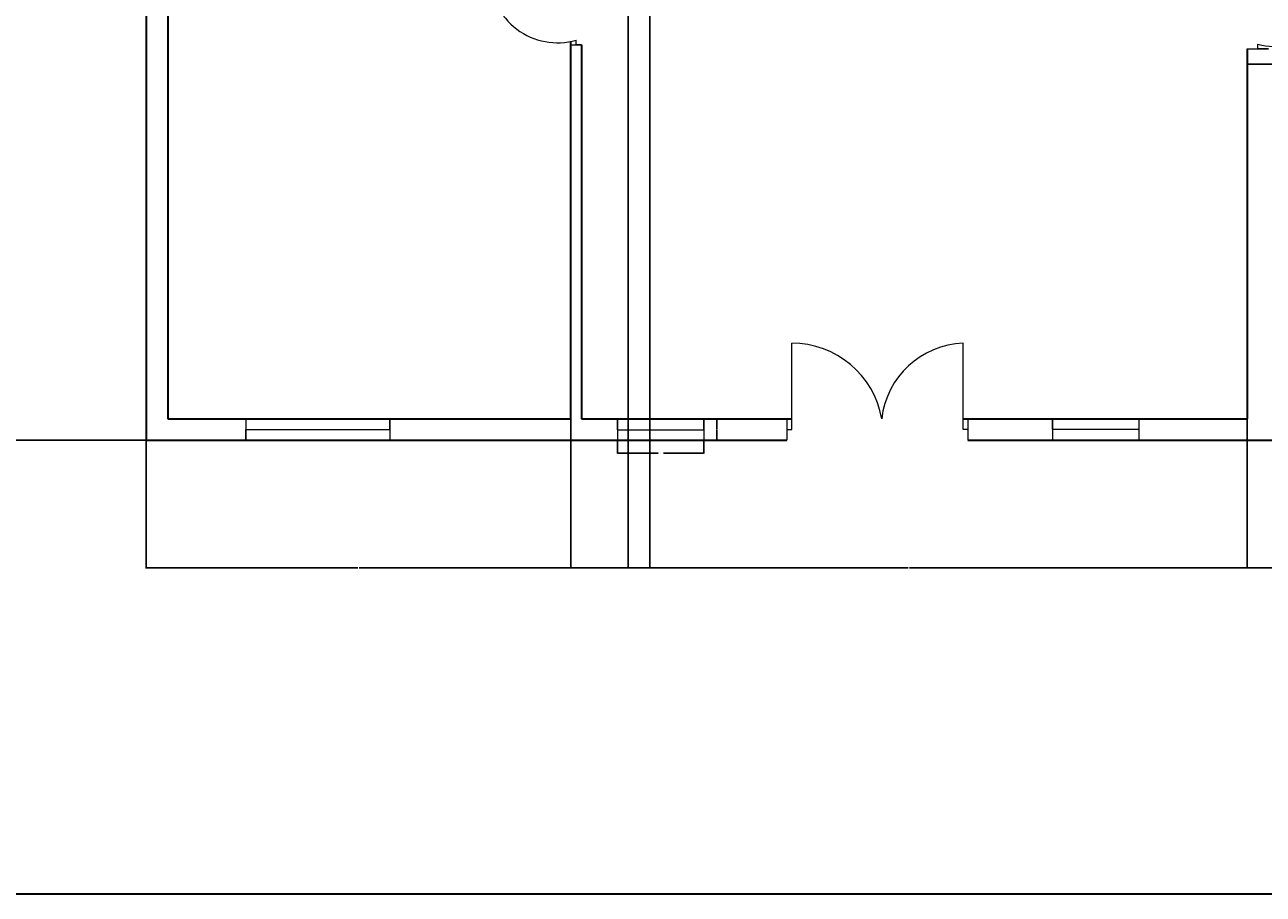
# Model space of a CAD drawing. Units: inches. Extents: x 2185 to 4426, y 1138 to 3073.
# Tile 8 of 14: x 3160 to 3677, y 1138 to 1501. Entities that reach past the tile are written whole.
import ezdxf

# ---------------------------------------------------------------- set-up
doc = ezdxf.new("R2010")
doc.units = ezdxf.units.IN
for name, color, linetype, lineweight in [('A-ANNO-DIMS', 2, 'Continuous', 18), ('A-ANNO-TTLB', 7, 'Continuous', 35), ('A-DOOR', 3, 'Continuous', 18), ('A-FURN', 8, 'Continuous', 18), ('A-GLAZ', 4, 'Continuous', 18), ('A-WALL', 7, 'Continuous', 35)]:
    doc.layers.add(name, color=color, linetype=linetype, lineweight=lineweight)
doc.styles.get("Standard").update_dxf_attribs({"font": 'arial.ttf'})
doc.dimstyles.get("Standard").update_dxf_attribs({"dimtxt": 0.18, "dimasz": 0.18, "dimexe": 0.18, "dimexo": 0.0625, "dimgap": 0.09, "dimtad": 0, "dimtih": 1, "dimtoh": 1, "dimdec": 4, "dimzin": 0, "dimdsep": 46, "dimtxsty": 'Standard', "dimcen": 0.09, "dimadec": 0, "dimazin": 0, "dimtfac": 1, "dimtdec": 4, "dimtofl": 0, "dimtmove": 0, "dimatfit": 3, "dimfxl": 1, "dimtolj": 1, "dimtzin": 0, "dimarcsym": 0})

# ---------------------------------------------------------------- blocks, each defined once
blk = doc.blocks.new('DOOR-SGL-36-BED-SW')
for p, q in [((38.25, 31.13), (33.75, 31.13)), ((33.75, 31.13), (36, 31.13)), ((36, 31.13), (36, 29.13)), ((36, 29.13), (0, 29.13)), ((36, 0), (36, 2)), ((33.75, 0), (38.25, 0)), ((38.25, 0), (36, 0))]:
    blk.add_line(p, q)
blk.add_arc((28.22, 29.13), 28.22, 180, 285.9925)
blk = doc.blocks.new('DOOR-PAIR-36-ENTRY')
for p, q in [((2, 4.5), (2, 40.5)), ((73.51, 4.5), (73.51, 40.5)), ((0, 9), (0, 0)), ((75.51, 9), (75.51, 0)), ((0, 4.5), (2, 4.5)), ((75.51, 4.5), (73.51, 4.5))]:
    blk.add_line(p, q)
for centre, radius, start, end in [((2, 2.35), 38.15, 10.036, 90), ((74.89, 4.97), 35.56, 92.226, 173.4897)]:
    blk.add_arc(centre, radius, start, end)
blk = doc.blocks.new('DOOR-SGL-36-BED-S')
for p, q in [((0, 31.73), (9, 31.73)), ((9, 31.73), (4.5, 31.73)), ((4.5, 31.73), (4.5, 31.73)), ((4.5, 31.73), (4.5, 29.73)), ((4.5, 29.73), (40.5, 29.73)), ((0, 0), (9, 0)), ((4.5, 0), (4.5, 2)), ((9, 0), (4.5, 0))]:
    blk.add_line(p, q)
blk.add_arc((11.82, 29.73), 28.68, 255.2109, 0)
blk = doc.blocks.new('WIN-PLAN-36IN-04')
for p, q in [((0, 4.34), (0, 9)), ((0, 9), (0, 0)), ((36, 4.34), (36, 9)), ((36, 9), (36, 9)), ((36, 9), (36, 0)), ((0, 4.34), (36, 4.34))]:
    blk.add_line(p, q)
blk = doc.blocks.new('WIN-PLAN-36IN-05')
for p, q in [((0, 4.66), (0, 9)), ((0, 9), (0, 0)), ((36, 9), (36, 0)), ((0, 4.66), (0, 4.66)), ((0, 4.66), (36, 4.66)), ((0, 4.66), (0, 4.66))]:
    blk.add_line(p, q)
blk = doc.blocks.new('WIN-PLAN-60IN-04')
for p, q in [((0, 9), (0, 0)), ((60, 4.5), (60, 9)), ((60, 9), (60, 0)), ((0, 0), (0, 4.5)), ((0, 4.5), (60, 4.5))]:
    blk.add_line(p, q)
blk = doc.blocks.new('*D90')
at = {"layer": 'A-ANNO-DIMS', "color": 0, "lineweight": -2, "transparency": 16777216}
for p, q in [((3669.85, 1490.29), (3669.85, 1484.1)), ((3710.35, 1490.29), (3710.35, 1484.1)), ((3670.03, 1484.28), (3689.16, 1484.28)), ((3710.17, 1484.28), (3691.03, 1484.28))]:
    blk.add_line(p, q, dxfattribs=at)
at = {"layer": 'A-ANNO-DIMS', "color": 0, "transparency": 16777216}
for points in [[(3670.03, 1484.31), (3670.03, 1484.25), (3669.85, 1484.28)], [(3710.17, 1484.31), (3710.17, 1484.25), (3710.35, 1484.28)]]:
    blk.add_solid(points, dxfattribs=at)
at = {"layer": 'Defpoints', "color": 0, "transparency": 16777216}
for p in [(3669.85, 1490.36), (3710.35, 1490.36), (3710.35, 1484.28)]:
    blk.add_point(p, dxfattribs=at)
at = {"layer": 'A-ANNO-DIMS', "color": 0, "transparency": 16777216, "insert": (3690.1, 1484.28), "char_height": 0.18, "attachment_point": 5}
blk.add_mtext('\\A1;DOOR 41 TYP.', dxfattribs=at)
blk = doc.blocks.new('*D98')
at = {"layer": 'A-ANNO-DIMS', "color": 0, "lineweight": -2, "transparency": 16777216}
for p, q in [((3407.37, 1327.31), (3407.37, 1321.8)), ((3443.37, 1327.31), (3443.37, 1321.8)), ((3407.55, 1321.98), (3424.25, 1321.98)), ((3443.19, 1321.98), (3426.49, 1321.98))]:
    blk.add_line(p, q, dxfattribs=at)
at = {"layer": 'A-ANNO-DIMS', "color": 0, "transparency": 16777216}
for points in [[(3407.55, 1322.01), (3407.55, 1321.95), (3407.37, 1321.98)], [(3443.19, 1322.01), (3443.19, 1321.95), (3443.37, 1321.98)]]:
    blk.add_solid(points, dxfattribs=at)
at = {"layer": 'Defpoints', "color": 0, "transparency": 16777216}
for p in [(3407.37, 1327.38), (3443.37, 1327.38), (3443.37, 1321.98)]:
    blk.add_point(p, dxfattribs=at)
at = {"layer": 'A-ANNO-DIMS', "color": 0, "transparency": 16777216, "insert": (3425.37, 1321.98), "char_height": 0.18, "attachment_point": 5}
blk.add_mtext('\\A1;WINDOW 36 TYP.', dxfattribs=at)
blk = doc.blocks.new('*D99')
at = {"layer": 'A-ANNO-DIMS', "color": 0, "lineweight": -2, "transparency": 16777216}
for p, q in [((3443.43, 1336.38), (3448.95, 1336.38)), ((3448.77, 1336.2), (3448.77, 1332.06)), ((3443.43, 1327.38), (3448.95, 1327.38)), ((3448.77, 1327.56), (3448.77, 1331.7))]:
    blk.add_line(p, q, dxfattribs=at)
at = {"layer": 'A-ANNO-DIMS', "color": 0, "transparency": 16777216}
for points in [[(3448.74, 1336.2), (3448.8, 1336.2), (3448.77, 1336.38)], [(3448.74, 1327.56), (3448.8, 1327.56), (3448.77, 1327.38)]]:
    blk.add_solid(points, dxfattribs=at)
at = {"layer": 'Defpoints', "color": 0, "transparency": 16777216}
for p in [(3443.37, 1336.38), (3448.77, 1336.38), (3443.37, 1327.38)]:
    blk.add_point(p, dxfattribs=at)
at = {"layer": 'A-ANNO-DIMS', "color": 0, "transparency": 16777216, "insert": (3448.77, 1331.88), "char_height": 0.18, "attachment_point": 5}
blk.add_mtext('\\A1;9 TYP.', dxfattribs=at)
blk = doc.blocks.new('*D147')
at = {"layer": 'A-ANNO-DIMS', "color": 0, "lineweight": -2, "transparency": 16777216}
for p, q in [((3387.85, 1336.31), (3387.85, 1273.95)), ((3210.85, 1327.31), (3210.85, 1273.95)), ((3211.03, 1274.13), (3299.07, 1274.13)), ((3387.67, 1274.13), (3299.63, 1274.13))]:
    blk.add_line(p, q, dxfattribs=at)
at = {"layer": 'A-ANNO-DIMS', "color": 0, "transparency": 16777216}
for points in [[(3211.03, 1274.16), (3211.03, 1274.1), (3210.85, 1274.13)], [(3387.67, 1274.16), (3387.67, 1274.1), (3387.85, 1274.13)]]:
    blk.add_solid(points, dxfattribs=at)
at = {"layer": 'Defpoints', "color": 0, "transparency": 16777216}
for p in [(3387.85, 1336.38), (3210.85, 1327.38), (3387.85, 1274.13)]:
    blk.add_point(p, dxfattribs=at)
at = {"layer": 'A-ANNO-DIMS', "color": 0, "transparency": 16777216, "insert": (3299.35, 1274.13), "char_height": 0.18, "attachment_point": 5}
blk.add_mtext('\\A1;177', dxfattribs=at)
blk = doc.blocks.new('*D148')
at = {"layer": 'A-ANNO-DIMS', "color": 0, "lineweight": -2, "transparency": 16777216}
for p, q in [((3387.85, 1336.31), (3387.85, 1273.95)), ((3669.85, 1336.31), (3669.85, 1273.95)), ((3388.03, 1274.13), (3528.56, 1274.13)), ((3669.67, 1274.13), (3529.14, 1274.13))]:
    blk.add_line(p, q, dxfattribs=at)
at = {"layer": 'A-ANNO-DIMS', "color": 0, "transparency": 16777216}
for points in [[(3388.03, 1274.16), (3388.03, 1274.1), (3387.85, 1274.13)], [(3669.67, 1274.16), (3669.67, 1274.1), (3669.85, 1274.13)]]:
    blk.add_solid(points, dxfattribs=at)
at = {"layer": 'Defpoints', "color": 0, "transparency": 16777216}
for p in [(3387.85, 1336.38), (3669.85, 1336.38), (3669.85, 1274.13)]:
    blk.add_point(p, dxfattribs=at)
at = {"layer": 'A-ANNO-DIMS', "color": 0, "transparency": 16777216, "insert": (3528.85, 1274.13), "char_height": 0.18, "attachment_point": 5}
blk.add_mtext('\\A1;282', dxfattribs=at)
blk = doc.blocks.new('*D149')
at = {"layer": 'A-ANNO-DIMS', "color": 0, "lineweight": -2, "transparency": 16777216}
for p, q in [((3669.85, 1336.31), (3669.85, 1273.95)), ((3932.35, 1327.31), (3932.35, 1273.95)), ((3670.03, 1274.13), (3800.7, 1274.13)), ((3932.17, 1274.13), (3801.5, 1274.13))]:
    blk.add_line(p, q, dxfattribs=at)
at = {"layer": 'A-ANNO-DIMS', "color": 0, "transparency": 16777216}
for points in [[(3670.03, 1274.16), (3670.03, 1274.1), (3669.85, 1274.13)], [(3932.17, 1274.16), (3932.17, 1274.1), (3932.35, 1274.13)]]:
    blk.add_solid(points, dxfattribs=at)
at = {"layer": 'Defpoints', "color": 0, "transparency": 16777216}
for p in [(3669.85, 1336.38), (3932.35, 1327.38), (3932.35, 1274.13)]:
    blk.add_point(p, dxfattribs=at)
at = {"layer": 'A-ANNO-DIMS', "color": 0, "transparency": 16777216, "insert": (3801.1, 1274.13), "char_height": 0.18, "attachment_point": 5}
blk.add_mtext('\\A1;262.5', dxfattribs=at)
blk = doc.blocks.new('*D150')
at = {"layer": 'A-ANNO-DIMS', "color": 0, "lineweight": -2, "transparency": 16777216}
for p, q in [((3219.79, 1528.38), (3101.64, 1528.38)), ((3101.82, 1528.2), (3101.82, 1428.06)), ((3101.82, 1327.56), (3101.82, 1427.7)), ((3210.79, 1327.38), (3101.64, 1327.38))]:
    blk.add_line(p, q, dxfattribs=at)
at = {"layer": 'A-ANNO-DIMS', "color": 0, "transparency": 16777216}
for points in [[(3101.79, 1528.2), (3101.85, 1528.2), (3101.82, 1528.38)], [(3101.79, 1327.56), (3101.85, 1327.56), (3101.82, 1327.38)]]:
    blk.add_solid(points, dxfattribs=at)
at = {"layer": 'Defpoints', "color": 0, "transparency": 16777216}
for p in [(3101.82, 1528.38), (3219.85, 1528.38), (3210.85, 1327.38)]:
    blk.add_point(p, dxfattribs=at)
at = {"layer": 'A-ANNO-DIMS', "color": 0, "transparency": 16777216, "insert": (3101.82, 1427.88), "char_height": 0.18, "attachment_point": 5}
blk.add_mtext('\\A1;201', dxfattribs=at)
blk = doc.blocks.new('*D161')
at = {"layer": 'A-ANNO-DIMS', "color": 0, "lineweight": -2, "transparency": 16777216}
for p, q in [((3420.81, 1609.31), (3420.81, 1273.95)), ((3411.81, 1600.31), (3411.81, 1273.95)), ((3411.99, 1274.13), (3416.16, 1274.13)), ((3420.63, 1274.13), (3416.46, 1274.13))]:
    blk.add_line(p, q, dxfattribs=at)
at = {"layer": 'A-ANNO-DIMS', "color": 0, "transparency": 16777216}
for points in [[(3411.99, 1274.16), (3411.99, 1274.1), (3411.81, 1274.13)], [(3420.63, 1274.16), (3420.63, 1274.1), (3420.81, 1274.13)]]:
    blk.add_solid(points, dxfattribs=at)
at = {"layer": 'Defpoints', "color": 0, "transparency": 16777216}
for p in [(3420.81, 1609.38), (3411.81, 1600.38), (3420.81, 1274.13)]:
    blk.add_point(p, dxfattribs=at)
at = {"layer": 'A-ANNO-DIMS', "color": 0, "transparency": 16777216, "insert": (3416.31, 1274.13), "char_height": 0.18, "attachment_point": 5}
blk.add_mtext('\\A1;9', dxfattribs=at)

msp = doc.modelspace()

# ---------------------------------------------------------------- linework, layer by layer
at = {"layer": 'A-ANNO-TTLB'}
msp.add_lwpolyline([(2184.741, 3073.364), (4426.252, 3073.364), (4426.252, 1137.99), (2184.741, 1137.99)], close=True, dxfattribs=at)
at = {"layer": 'A-FURN'}
for p, q in [((3219.849, 1459.067), (3219.849, 1459.485)), ((3219.849, 1459.067), (3219.849, 1459.485)), ((3219.849, 1371.675), (3219.849, 1459.067)), ((3219.849, 1371.675), (3219.849, 1459.067))]:
    msp.add_line(p, q, dxfattribs=at)
at = {"layer": 'A-WALL'}
for p, q in [((3210.849, 2136.303), (3210.849, 1327.377)), ((3210.849, 2136.303), (3210.849, 1327.377)), ((3210.849, 2136.303), (3210.849, 1327.377)), ((3210.849, 2136.303), (3210.849, 1327.377)), ((3219.849, 1528.377), (3219.849, 1336.377)), ((3219.849, 1528.377), (3219.849, 1336.377)), ((3219.849, 1528.377), (3219.849, 1336.377)), ((3219.849, 1528.377), (3219.849, 1336.377)), ((3387.849, 1336.377), (3387.849, 1493.761)), ((3387.849, 1336.377), (3387.849, 1493.761)), ((3392.349, 1492.307), (3392.349, 1336.377)), ((3392.349, 1492.307), (3392.349, 1336.377)), ((3669.849, 1490.627), (3669.849, 1336.377)), ((3669.849, 1490.627), (3669.849, 1336.377)), ((3219.849, 1336.377), (3387.849, 1336.377)), ((3219.849, 1336.377), (3387.849, 1336.377)), ((3219.849, 1336.377), (3387.849, 1336.377)), ((3219.849, 1336.377), (3387.849, 1336.377)), ((3392.349, 1336.377), (3479.974, 1336.377)), ((3392.349, 1336.377), (3479.974, 1336.377)), ((3443.369, 1336.377), (3479.974, 1336.377)), ((3443.369, 1336.377), (3479.974, 1336.377)), ((3551.486, 1336.377), (3669.849, 1336.377)), ((3551.486, 1336.377), (3669.849, 1336.377)), ((3210.849, 1327.377), (3477.974, 1327.377)), ((3210.849, 1327.377), (3477.974, 1327.377)), ((3443.369, 1327.377), (3477.974, 1327.377)), ((3443.369, 1327.377), (3477.974, 1327.377)), ((3553.486, 1327.377), (3932.349, 1327.377)), ((3553.486, 1327.377), (3932.349, 1327.377))]:
    msp.add_line(p, q, dxfattribs=at)

# ---------------------------------------------------------------- block references
at = {"layer": 'A-DOOR'}
for name, p in [('DOOR-SGL-36-BED-SW', (3354.099, 1492.307)), ('DOOR-SGL-36-BED-SW', (3354.099, 1492.307)), ('DOOR-SGL-36-BED-S', (3669.849, 1490.627)), ('DOOR-SGL-36-BED-S', (3669.849, 1490.627)), ('DOOR-PAIR-36-ENTRY', (3477.974, 1327.377)), ('DOOR-PAIR-36-ENTRY', (3477.974, 1327.377))]:
    msp.add_blockref(name, p, dxfattribs=at)
at = {"layer": 'A-GLAZ'}
for name, p in [('WIN-PLAN-60IN-04', (3252.369, 1327.377)), ('WIN-PLAN-60IN-04', (3252.369, 1327.377)), ('WIN-PLAN-36IN-04', (3407.369, 1327.377)), ('WIN-PLAN-36IN-04', (3407.369, 1327.377)), ('WIN-PLAN-36IN-05', (3588.761, 1327.377)), ('WIN-PLAN-36IN-05', (3588.761, 1327.377))]:
    msp.add_blockref(name, p, dxfattribs=at)

# ---------------------------------------------------------------- dimensions: what is measured, and where the dimension line sits
at = {"layer": 'A-ANNO-DIMS'}
for base, p1, p2, override, picture, middle in [((3420.807, 1274.127), (3411.807, 1600.377), (3420.807, 1609.377), {"dimdec": 0, "dimlfac": 1, "dimrnd": 0, "dimzin": 0, "dimdsep": 46, "dimlunit": 2}, '*D161', (3416.307, 1274.127)), ((3387.849, 1274.127), (3210.849, 1327.377), (3387.849, 1336.377), {"dimdec": 0, "dimlfac": 1, "dimrnd": 0, "dimzin": 0, "dimdsep": 46, "dimlunit": 2}, '*D147', (3299.349, 1274.127)), ((3669.849, 1274.127), (3387.849, 1336.377), (3669.849, 1336.377), {"dimdec": 0, "dimlfac": 1, "dimrnd": 0, "dimzin": 0, "dimdsep": 46, "dimlunit": 2}, '*D148', (3528.849, 1274.127)), ((3932.349, 1274.127), (3669.849, 1336.377), (3932.349, 1327.377), {"dimdec": 1, "dimlfac": 1, "dimrnd": 0, "dimzin": 0, "dimdsep": 46, "dimlunit": 2}, '*D149', (3801.099, 1274.127))]:
    dim = msp.add_linear_dim(base=base, p1=p1, p2=p2, dimstyle='Standard', override=override, dxfattribs=at)
    dim.commit()
    dim.dimension.update_dxf_attribs({"geometry": picture, "text_midpoint": middle})
dim = msp.add_linear_dim(base=(3101.824, 1528.377), p1=(3210.849, 1327.377), p2=(3219.849, 1528.377), angle=90, dimstyle='Standard', override={"dimdec": 0, "dimlfac": 1, "dimrnd": 0, "dimzin": 0, "dimdsep": 46, "dimlunit": 2}, dxfattribs=at)
dim.commit()
dim.dimension.update_dxf_attribs({"geometry": '*D150', "text_midpoint": (3101.824, 1427.877)})
for base, p1, p2, text, picture, middle in [((3710.34919158, 1484.281003331), (3669.84919158, 1490.356003331), (3710.34919158, 1490.356003331), 'DOOR <> TYP.', '*D90', (3690.09919158, 1484.281003331)), ((3443.369, 1321.977), (3407.369, 1327.377), (3443.369, 1327.377), 'WINDOW <> TYP.', '*D98', (3425.369, 1321.977))]:
    dim = msp.add_linear_dim(base=base, p1=p1, p2=p2, text=text, dimstyle='Standard', override={"dimdec": 0, "dimlfac": 1, "dimrnd": 0, "dimzin": 0, "dimdsep": 46, "dimlunit": 2}, dxfattribs=at)
    dim.commit()
    dim.dimension.update_dxf_attribs({"geometry": picture, "text_midpoint": middle})
dim = msp.add_linear_dim(base=(3448.769, 1336.377), p1=(3443.369, 1327.377), p2=(3443.369, 1336.377), angle=90, text='<> TYP.', dimstyle='Standard', override={"dimdec": 0, "dimlfac": 1, "dimrnd": 0, "dimzin": 0, "dimdsep": 46, "dimlunit": 2}, dxfattribs=at)
dim.commit()
dim.dimension.update_dxf_attribs({"geometry": '*D99', "text_midpoint": (3448.769, 1331.877)})

doc.saveas('drawing.dxf')
